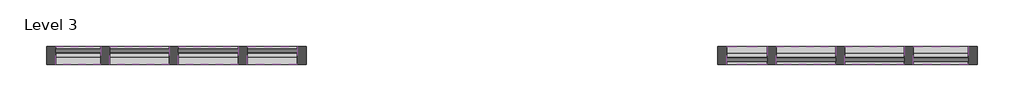
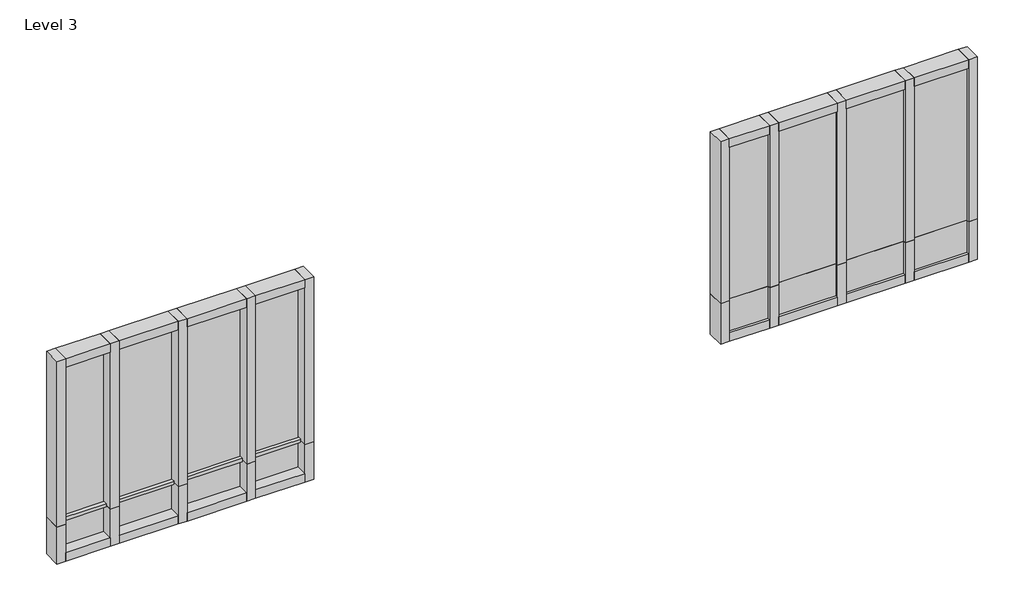
# One storey, incomplete: 44 members, 16 plates.
"""IFC4 building model written with IfcOpenShell, lengths in millimetres."""

from ifc_helpers import new_model, si_unit, origin, place, context, project, spatial, transform, mapped, element, save
from components import member_2ec808cb, member_7ddf0b01, member_ff98d70f, member_bdd069ac, member_fa046a42, member_66d82eec, member_4918008d, member_3060f3e2, member_6be37683, member_ccaabd6e, member_6ea553f1, member_a1da5be3, member_71eb4692, member_d3323a85, member_6c34f49c, member_dffdf235, member_75d1e245, member_2b49869a, member_75074519, member_3c3dc66a, system_panel_glazed_5633d65b, system_panel_glazed_b006000b, system_panel_glazed_54f7da7e, system_panel_glazed_325805c1, system_panel_glazed_de0a1ab2, system_panel_glazed_75a4b6fa, system_panel_glazed_925bd09e, system_panel_glazed_45aa6f3c, system_panel_glazed_e947191b, system_panel_glazed_5768b914, system_panel_glazed_0f3faf12, system_panel_glazed_eddfd4ea, system_panel_glazed_fe17e9eb, system_panel_glazed_f0550140

model = new_model("IFC4")

# Units and contexts
model_context = context("Model", 3, world=origin())
ifc_project = project(units=[si_unit("LENGTHUNIT", "METRE", prefix="MILLI")], contexts=[model_context])

# Site, building, storey
site = spatial("IfcSite", under=ifc_project)
building = spatial("IfcBuilding", under=site)
storey = spatial("IfcBuildingStorey", under=building, Name="Level 3", Elevation=3200.4)

# Members
placement = place(None, origin())
member_shape = member_2ec808cb(model_context)
element("IfcMember", 1, ObjectType="Rectangular Mullion : 1\" Square", at=placement, inside=storey, context=model_context, shape_type="MappedRepresentation", body=[
    mapped(member_shape, transform((-4793.1680265, 1641.9286055, 4089.4), x_axis=(0.0, 0.0, 1.0), y_axis=(0.0, -1.0, 0.0), z_axis=(1.0, 0.0, 0.0))),
])
member_2_shape = member_7ddf0b01(model_context)
element("IfcMember", 2, ObjectType="Rectangular Mullion : 1\" Square", at=placement, inside=storey, context=model_context, shape_type="MappedRepresentation", body=[
    mapped(member_2_shape, transform((-5208.0346932, 1641.9286055, 4089.4), x_axis=(0.0, 0.0, 1.0), y_axis=(0.0, -1.0, 0.0), z_axis=(1.0, 0.0, 0.0))),
])
member_3_shape = member_ff98d70f(model_context)
element("IfcMember", 3, ObjectType="Rectangular Mullion : 1\" Square", at=placement, inside=storey, context=model_context, shape_type="MappedRepresentation", body=[
    mapped(member_3_shape, transform((-5694.8680265, 1641.9286055, 4089.4), x_axis=(0.0, 0.0, 1.0), y_axis=(0.0, -1.0, 0.0), z_axis=(1.0, 0.0, 0.0))),
])
element("IfcMember", 4, ObjectType="Rectangular Mullion : 1\" Square", at=placement, inside=storey, context=model_context, shape_type="MappedRepresentation", body=[
    mapped(member_3_shape, transform((-938.7180265, 1641.9286055, 4114.8), x_axis=(0.0, 0.0, 1.0), y_axis=(0.0, 1.0, 0.0), z_axis=(-1.0, 0.0, 0.0))),
])
element("IfcMember", 5, ObjectType="Rectangular Mullion : 1\" Square", at=placement, inside=storey, context=model_context, shape_type="MappedRepresentation", body=[
    mapped(member_3_shape, transform((-1421.3180265, 1641.9286055, 4114.8), x_axis=(0.0, 0.0, 1.0), y_axis=(0.0, 1.0, 0.0), z_axis=(-1.0, 0.0, 0.0))),
])
member_4_shape = member_bdd069ac(model_context)
element("IfcMember", 6, ObjectType="Rectangular Mullion : 1\" Square", at=placement, inside=storey, context=model_context, shape_type="MappedRepresentation", body=[
    mapped(member_4_shape, transform((-6177.4680265, 1641.9286055, 4089.4), x_axis=(0.0, 0.0, 1.0), y_axis=(0.0, -1.0, 0.0), z_axis=(1.0, 0.0, 0.0))),
])
member_5_shape = member_fa046a42(model_context)
element("IfcMember", 7, ObjectType="Rectangular Mullion : 1\" Square", at=placement, inside=storey, context=model_context, shape_type="MappedRepresentation", body=[
    mapped(member_5_shape, transform((-1770.5680265, 1641.9286055, 4114.8), x_axis=(0.0, 0.0, 1.0), y_axis=(0.0, 1.0, 0.0), z_axis=(-1.0, 0.0, 0.0))),
])
member_6_shape = member_66d82eec(model_context)
element("IfcMember", 8, ObjectType="Rectangular Mullion : 1\" Square", at=placement, inside=storey, context=model_context, shape_type="MappedRepresentation", body=[
    mapped(member_6_shape, transform((-456.1180265, 1641.9286055, 4114.8), x_axis=(0.0, 0.0, 1.0), y_axis=(0.0, 1.0, 0.0), z_axis=(-1.0, 0.0, 0.0))),
])
member_7_shape = member_4918008d(model_context)
element("IfcMember", 9, ObjectType="Rectangular Mullion : 2.5\" x 5\" rectangular", at=placement, inside=storey, context=model_context, shape_type="MappedRepresentation", body=[
    mapped(member_7_shape, transform((-4793.1680265, 1641.9286055, 5334.0), x_axis=(0.0, 0.0, 1.0), y_axis=(0.0, -1.0, 0.0), z_axis=(1.0, 0.0, 0.0))),
])
member_8_shape = member_3060f3e2(model_context)
element("IfcMember", 10, ObjectType="Rectangular Mullion : 2.5\" x 5\" rectangular", at=placement, inside=storey, context=model_context, shape_type="MappedRepresentation", body=[
    mapped(member_8_shape, transform((-6494.9680265, 1641.9286055, 3810.0), x_axis=(0.0, 0.0, -1.0), y_axis=(0.0, -1.0, 0.0), z_axis=(-1.0, 0.0, 0.0))),
])
member_9_shape = member_6be37683(model_context)
element("IfcMember", 11, ObjectType="Rectangular Mullion : 2.5\" x 5\" rectangular", at=placement, inside=storey, context=model_context, shape_type="MappedRepresentation", body=[
    mapped(member_9_shape, transform((-6145.7180265, 1641.9286055, 3810.0), x_axis=(1.0, 0.0, 0.0), y_axis=(0.0, -1.0, 0.0), z_axis=(0.0, 0.0, -1.0))),
])
element("IfcMember", 12, ObjectType="Rectangular Mullion : 2.5\" x 5\" rectangular", at=placement, inside=storey, context=model_context, shape_type="MappedRepresentation", body=[
    mapped(member_9_shape, transform((-5663.1180265, 1641.9286055, 3810.0), x_axis=(1.0, 0.0, 0.0), y_axis=(0.0, -1.0, 0.0), z_axis=(0.0, 0.0, -1.0))),
])
element("IfcMember", 13, ObjectType="Rectangular Mullion : 2.5\" x 5\" rectangular", at=placement, inside=storey, context=model_context, shape_type="MappedRepresentation", body=[
    mapped(member_9_shape, transform((-5176.2846932, 1641.9286055, 3810.0), x_axis=(1.0, 0.0, 0.0), y_axis=(0.0, -1.0, 0.0), z_axis=(0.0, 0.0, -1.0))),
])
member_10_shape = member_ccaabd6e(model_context)
element("IfcMember", 14, ObjectType="Rectangular Mullion : 2.5\" x 5\" rectangular", at=placement, inside=storey, context=model_context, shape_type="MappedRepresentation", body=[
    mapped(member_10_shape, transform((-6113.9680265, 1641.9286055, 3810.0), x_axis=(0.0, 0.0, -1.0), y_axis=(0.0, -1.0, 0.0), z_axis=(-1.0, 0.0, 0.0))),
])
element("IfcMember", 15, ObjectType="Rectangular Mullion : 2.5\" x 5\" rectangular", at=placement, inside=storey, context=model_context, shape_type="MappedRepresentation", body=[
    mapped(member_10_shape, transform((-1002.2180265, 1641.9286055, 3810.0), x_axis=(0.0, 0.0, -1.0), y_axis=(0.0, 1.0, 0.0), z_axis=(1.0, 0.0, 0.0))),
])
element("IfcMember", 16, ObjectType="Rectangular Mullion : 2.5\" x 5\" rectangular", at=placement, inside=storey, context=model_context, shape_type="MappedRepresentation", body=[
    mapped(member_10_shape, transform((-519.6180265, 1641.9286055, 3810.0), x_axis=(0.0, 0.0, -1.0), y_axis=(0.0, 1.0, 0.0), z_axis=(1.0, 0.0, 0.0))),
])
member_11_shape = member_6ea553f1(model_context)
element("IfcMember", 17, ObjectType="Rectangular Mullion : 2.5\" x 5\" rectangular", at=placement, inside=storey, context=model_context, shape_type="MappedRepresentation", body=[
    mapped(member_11_shape, transform((-5631.3680265, 1641.9286055, 3810.0), x_axis=(0.0, 0.0, -1.0), y_axis=(0.0, -1.0, 0.0), z_axis=(-1.0, 0.0, 0.0))),
])
element("IfcMember", 18, ObjectType="Rectangular Mullion : 2.5\" x 5\" rectangular", at=placement, inside=storey, context=model_context, shape_type="MappedRepresentation", body=[
    mapped(member_7_shape, transform((-5144.5346932, 1641.9286055, 3810.0), x_axis=(0.0, 0.0, -1.0), y_axis=(0.0, -1.0, 0.0), z_axis=(-1.0, 0.0, 0.0))),
])
element("IfcMember", 19, ObjectType="Rectangular Mullion : 2.5\" x 5\" rectangular", at=placement, inside=storey, context=model_context, shape_type="MappedRepresentation", body=[
    mapped(member_8_shape, transform((-6177.4680265, 1641.9286055, 5334.0), x_axis=(0.0, 0.0, 1.0), y_axis=(0.0, -1.0, 0.0), z_axis=(1.0, 0.0, 0.0))),
])
element("IfcMember", 20, ObjectType="Rectangular Mullion : 2.5\" x 5\" rectangular", at=placement, inside=storey, context=model_context, shape_type="MappedRepresentation", body=[
    mapped(member_10_shape, transform((-5694.8680265, 1641.9286055, 5334.0), x_axis=(0.0, 0.0, 1.0), y_axis=(0.0, -1.0, 0.0), z_axis=(1.0, 0.0, 0.0))),
])
element("IfcMember", 21, ObjectType="Rectangular Mullion : 2.5\" x 5\" rectangular", at=placement, inside=storey, context=model_context, shape_type="MappedRepresentation", body=[
    mapped(member_10_shape, transform((-1421.3180265, 1641.9286055, 5334.0), x_axis=(0.0, 0.0, 1.0), y_axis=(0.0, 1.0, 0.0), z_axis=(-1.0, 0.0, 0.0))),
])
element("IfcMember", 22, ObjectType="Rectangular Mullion : 2.5\" x 5\" rectangular", at=placement, inside=storey, context=model_context, shape_type="MappedRepresentation", body=[
    mapped(member_10_shape, transform((-938.7180265, 1641.9286055, 5334.0), x_axis=(0.0, 0.0, 1.0), y_axis=(0.0, 1.0, 0.0), z_axis=(-1.0, 0.0, 0.0))),
])
element("IfcMember", 23, ObjectType="Rectangular Mullion : 2.5\" x 5\" rectangular", at=placement, inside=storey, context=model_context, shape_type="MappedRepresentation", body=[
    mapped(member_11_shape, transform((-5208.0346932, 1641.9286055, 5334.0), x_axis=(0.0, 0.0, 1.0), y_axis=(0.0, -1.0, 0.0), z_axis=(1.0, 0.0, 0.0))),
])
member_12_shape = member_a1da5be3(model_context)
element("IfcMember", 24, ObjectType="Rectangular Mullion : 2.5\" x 5\" rectangular", at=placement, inside=storey, context=model_context, shape_type="MappedRepresentation", body=[
    mapped(member_12_shape, transform((-6145.7180265, 1641.9286055, 4089.4), x_axis=(1.0, 0.0, 0.0), y_axis=(0.0, -1.0, 0.0), z_axis=(0.0, 0.0, -1.0))),
])
element("IfcMember", 25, ObjectType="Rectangular Mullion : 2.5\" x 5\" rectangular", at=placement, inside=storey, context=model_context, shape_type="MappedRepresentation", body=[
    mapped(member_12_shape, transform((-5663.1180265, 1641.9286055, 4089.4), x_axis=(1.0, 0.0, 0.0), y_axis=(0.0, -1.0, 0.0), z_axis=(0.0, 0.0, -1.0))),
])
element("IfcMember", 26, ObjectType="Rectangular Mullion : 2.5\" x 5\" rectangular", at=placement, inside=storey, context=model_context, shape_type="MappedRepresentation", body=[
    mapped(member_12_shape, transform((-5176.2846932, 1641.9286055, 4089.4), x_axis=(1.0, 0.0, 0.0), y_axis=(0.0, -1.0, 0.0), z_axis=(0.0, 0.0, -1.0))),
])
member_13_shape = member_71eb4692(model_context)
element("IfcMember", 27, ObjectType="Rectangular Mullion : 2.5\" x 5\" rectangular", at=placement, inside=storey, context=model_context, shape_type="MappedRepresentation", body=[
    mapped(member_13_shape, transform((-6558.4680265, 1641.9286055, 5334.0), x_axis=(-1.0, 0.0, 0.0), y_axis=(0.0, -1.0, 0.0), z_axis=(0.0, 0.0, 1.0))),
])
member_14_shape = member_d3323a85(model_context)
element("IfcMember", 28, ObjectType="Rectangular Mullion : 2.5\" x 5\" rectangular", at=placement, inside=storey, context=model_context, shape_type="MappedRepresentation", body=[
    mapped(member_14_shape, transform((-4729.6680265, 1641.9286055, 3810.0), x_axis=(1.0, 0.0, 0.0), y_axis=(0.0, -1.0, 0.0), z_axis=(0.0, 0.0, -1.0))),
])
element("IfcMember", 29, ObjectType="Rectangular Mullion : 2.5\" x 5\" rectangular", at=placement, inside=storey, context=model_context, shape_type="MappedRepresentation", body=[
    mapped(member_13_shape, transform((-4729.6680265, 1641.9286055, 4089.4), x_axis=(1.0, 0.0, 0.0), y_axis=(0.0, -1.0, 0.0), z_axis=(0.0, 0.0, -1.0))),
])
element("IfcMember", 30, ObjectType="Rectangular Mullion : 2.5\" x 5\" rectangular", at=placement, inside=storey, context=model_context, shape_type="MappedRepresentation", body=[
    mapped(member_14_shape, transform((-6558.4680265, 1641.9286055, 4089.4), x_axis=(-1.0, 0.0, 0.0), y_axis=(0.0, -1.0, 0.0), z_axis=(0.0, 0.0, 1.0))),
])
member_15_shape = member_6c34f49c(model_context)
element("IfcMember", 31, ObjectType="Rectangular Mullion : 2.5\" x 5\" rectangular", at=placement, inside=storey, context=model_context, shape_type="MappedRepresentation", body=[
    mapped(member_15_shape, transform((-1770.5680265, 1641.9286055, 5334.0), x_axis=(0.0, 0.0, 1.0), y_axis=(0.0, 1.0, 0.0), z_axis=(-1.0, 0.0, 0.0))),
])
member_16_shape = member_dffdf235(model_context)
element("IfcMember", 32, ObjectType="Rectangular Mullion : 2.5\" x 5\" rectangular", at=placement, inside=storey, context=model_context, shape_type="MappedRepresentation", body=[
    mapped(member_16_shape, transform((-68.7680265, 1641.9286055, 3810.0), x_axis=(0.0, 0.0, -1.0), y_axis=(0.0, 1.0, 0.0), z_axis=(1.0, 0.0, 0.0))),
])
member_17_shape = member_75d1e245(model_context)
element("IfcMember", 33, ObjectType="Rectangular Mullion : 2.5\" x 5\" rectangular", at=placement, inside=storey, context=model_context, shape_type="MappedRepresentation", body=[
    mapped(member_17_shape, transform((-1453.0680265, 1641.9286055, 3810.0), x_axis=(-1.0, 0.0, 0.0), y_axis=(0.0, 1.0, 0.0), z_axis=(0.0, 0.0, -1.0))),
])
element("IfcMember", 34, ObjectType="Rectangular Mullion : 2.5\" x 5\" rectangular", at=placement, inside=storey, context=model_context, shape_type="MappedRepresentation", body=[
    mapped(member_17_shape, transform((-970.4680265, 1641.9286055, 3810.0), x_axis=(-1.0, 0.0, 0.0), y_axis=(0.0, 1.0, 0.0), z_axis=(0.0, 0.0, -1.0))),
])
element("IfcMember", 35, ObjectType="Rectangular Mullion : 2.5\" x 5\" rectangular", at=placement, inside=storey, context=model_context, shape_type="MappedRepresentation", body=[
    mapped(member_17_shape, transform((-487.8680265, 1641.9286055, 3810.0), x_axis=(-1.0, 0.0, 0.0), y_axis=(0.0, 1.0, 0.0), z_axis=(0.0, 0.0, -1.0))),
])
element("IfcMember", 36, ObjectType="Rectangular Mullion : 2.5\" x 5\" rectangular", at=placement, inside=storey, context=model_context, shape_type="MappedRepresentation", body=[
    mapped(member_15_shape, transform((-1484.8180265, 1641.9286055, 3810.0), x_axis=(0.0, 0.0, -1.0), y_axis=(0.0, 1.0, 0.0), z_axis=(1.0, 0.0, 0.0))),
])
element("IfcMember", 37, ObjectType="Rectangular Mullion : 2.5\" x 5\" rectangular", at=placement, inside=storey, context=model_context, shape_type="MappedRepresentation", body=[
    mapped(member_16_shape, transform((-456.1180265, 1641.9286055, 5334.0), x_axis=(0.0, 0.0, 1.0), y_axis=(0.0, 1.0, 0.0), z_axis=(-1.0, 0.0, 0.0))),
])
member_18_shape = member_2b49869a(model_context)
element("IfcMember", 38, ObjectType="Rectangular Mullion : 2.5\" x 5\" rectangular", at=placement, inside=storey, context=model_context, shape_type="MappedRepresentation", body=[
    mapped(member_18_shape, transform((-1453.0680265, 1641.9286055, 4114.8), x_axis=(-1.0, 0.0, 0.0), y_axis=(0.0, 1.0, 0.0), z_axis=(0.0, 0.0, -1.0))),
])
element("IfcMember", 39, ObjectType="Rectangular Mullion : 2.5\" x 5\" rectangular", at=placement, inside=storey, context=model_context, shape_type="MappedRepresentation", body=[
    mapped(member_18_shape, transform((-970.4680265, 1641.9286055, 4114.8), x_axis=(-1.0, 0.0, 0.0), y_axis=(0.0, 1.0, 0.0), z_axis=(0.0, 0.0, -1.0))),
])
element("IfcMember", 40, ObjectType="Rectangular Mullion : 2.5\" x 5\" rectangular", at=placement, inside=storey, context=model_context, shape_type="MappedRepresentation", body=[
    mapped(member_18_shape, transform((-487.8680265, 1641.9286055, 4114.8), x_axis=(-1.0, 0.0, 0.0), y_axis=(0.0, 1.0, 0.0), z_axis=(0.0, 0.0, -1.0))),
])
member_19_shape = member_75074519(model_context)
element("IfcMember", 41, ObjectType="Rectangular Mullion : 2.5\" x 5\" rectangular", at=placement, inside=storey, context=model_context, shape_type="MappedRepresentation", body=[
    mapped(member_19_shape, transform((-5.2680265, 1641.9286055, 5334.0), x_axis=(1.0, 0.0, 0.0), y_axis=(0.0, 1.0, 0.0), z_axis=(0.0, 0.0, 1.0))),
])
member_20_shape = member_3c3dc66a(model_context)
element("IfcMember", 42, ObjectType="Rectangular Mullion : 2.5\" x 5\" rectangular", at=placement, inside=storey, context=model_context, shape_type="MappedRepresentation", body=[
    mapped(member_20_shape, transform((-1834.0680265, 1641.9286055, 3810.0), x_axis=(-1.0, 0.0, 0.0), y_axis=(0.0, 1.0, 0.0), z_axis=(0.0, 0.0, -1.0))),
])
element("IfcMember", 43, ObjectType="Rectangular Mullion : 2.5\" x 5\" rectangular", at=placement, inside=storey, context=model_context, shape_type="MappedRepresentation", body=[
    mapped(member_19_shape, transform((-1834.0680265, 1641.9286055, 4114.8), x_axis=(-1.0, 0.0, 0.0), y_axis=(0.0, 1.0, 0.0), z_axis=(0.0, 0.0, -1.0))),
])
element("IfcMember", 44, ObjectType="Rectangular Mullion : 2.5\" x 5\" rectangular", at=placement, inside=storey, context=model_context, shape_type="MappedRepresentation", body=[
    mapped(member_20_shape, transform((-5.2680265, 1641.9286055, 4114.8), x_axis=(1.0, 0.0, 0.0), y_axis=(0.0, 1.0, 0.0), z_axis=(0.0, 0.0, 1.0))),
])

# Plates
system_panel_glazed_shape = system_panel_glazed_5633d65b(model_context)
element("IfcPlate", 45, ObjectType="System Panel : Glazed", at=placement, inside=storey, context=model_context, shape_type="MappedRepresentation", body=[
    mapped(system_panel_glazed_shape, transform((-6336.2180265, 1641.9286055, 3873.5), x_axis=(1.0, 0.0, 0.0), y_axis=(0.0, 1.0, 0.0), z_axis=(0.0, 0.0, 1.0))),
])
system_panel_glazed_2_shape = system_panel_glazed_b006000b(model_context)
element("IfcPlate", 46, ObjectType="System Panel : Glazed", at=placement, inside=storey, context=model_context, shape_type="MappedRepresentation", body=[
    mapped(system_panel_glazed_2_shape, transform((-5904.4180265, 1641.9286055, 3873.5), x_axis=(1.0, 0.0, 0.0), y_axis=(0.0, 1.0, 0.0), z_axis=(0.0, 0.0, 1.0))),
])
system_panel_glazed_3_shape = system_panel_glazed_54f7da7e(model_context)
element("IfcPlate", 47, ObjectType="System Panel : Glazed", at=placement, inside=storey, context=model_context, shape_type="MappedRepresentation", body=[
    mapped(system_panel_glazed_3_shape, transform((-5419.7013599, 1641.9286055, 3873.5), x_axis=(1.0, 0.0, 0.0), y_axis=(0.0, 1.0, 0.0), z_axis=(0.0, 0.0, 1.0))),
])
system_panel_glazed_4_shape = system_panel_glazed_325805c1(model_context)
element("IfcPlate", 48, ObjectType="System Panel : Glazed", at=placement, inside=storey, context=model_context, shape_type="MappedRepresentation", body=[
    mapped(system_panel_glazed_4_shape, transform((-4968.8513599, 1641.9286055, 3873.5), x_axis=(1.0, 0.0, 0.0), y_axis=(0.0, 1.0, 0.0), z_axis=(0.0, 0.0, 1.0))),
])
system_panel_glazed_5_shape = system_panel_glazed_de0a1ab2(model_context)
element("IfcPlate", 49, ObjectType="System Panel : Glazed", at=placement, inside=storey, context=model_context, shape_type="MappedRepresentation", body=[
    mapped(system_panel_glazed_5_shape, transform((-6336.2180265, 1641.9286055, 4089.4), x_axis=(1.0, 0.0, 0.0), y_axis=(0.0, 1.0, 0.0), z_axis=(0.0, 0.0, 1.0))),
])
system_panel_glazed_6_shape = system_panel_glazed_75a4b6fa(model_context)
element("IfcPlate", 50, ObjectType="System Panel : Glazed", at=placement, inside=storey, context=model_context, shape_type="MappedRepresentation", body=[
    mapped(system_panel_glazed_6_shape, transform((-5904.4180265, 1641.9286055, 4089.4), x_axis=(1.0, 0.0, 0.0), y_axis=(0.0, 1.0, 0.0), z_axis=(0.0, 0.0, 1.0))),
])
system_panel_glazed_7_shape = system_panel_glazed_925bd09e(model_context)
element("IfcPlate", 51, ObjectType="System Panel : Glazed", at=placement, inside=storey, context=model_context, shape_type="MappedRepresentation", body=[
    mapped(system_panel_glazed_7_shape, transform((-5419.7013599, 1641.9286055, 4089.4), x_axis=(1.0, 0.0, 0.0), y_axis=(0.0, 1.0, 0.0), z_axis=(0.0, 0.0, 1.0))),
])
system_panel_glazed_8_shape = system_panel_glazed_45aa6f3c(model_context)
element("IfcPlate", 52, ObjectType="System Panel : Glazed", at=placement, inside=storey, context=model_context, shape_type="MappedRepresentation", body=[
    mapped(system_panel_glazed_8_shape, transform((-4968.8513599, 1641.9286055, 4089.4), x_axis=(1.0, 0.0, 0.0), y_axis=(0.0, 1.0, 0.0), z_axis=(0.0, 0.0, 1.0))),
])
system_panel_glazed_9_shape = system_panel_glazed_e947191b(model_context)
element("IfcPlate", 53, ObjectType="System Panel : Glazed", at=placement, inside=storey, context=model_context, shape_type="MappedRepresentation", body=[
    mapped(system_panel_glazed_9_shape, transform((-262.4430265, 1641.9286055, 3873.5), x_axis=(-1.0, 0.0, 0.0), y_axis=(0.0, -1.0, 0.0), z_axis=(0.0, 0.0, 1.0))),
])
system_panel_glazed_10_shape = system_panel_glazed_5768b914(model_context)
element("IfcPlate", 54, ObjectType="System Panel : Glazed", at=placement, inside=storey, context=model_context, shape_type="MappedRepresentation", body=[
    mapped(system_panel_glazed_10_shape, transform((-1627.6930265, 1641.9286055, 3873.5), x_axis=(-1.0, 0.0, 0.0), y_axis=(0.0, -1.0, 0.0), z_axis=(0.0, 0.0, 1.0))),
])
system_panel_glazed_11_shape = system_panel_glazed_0f3faf12(model_context)
element("IfcPlate", 55, ObjectType="System Panel : Glazed", at=placement, inside=storey, context=model_context, shape_type="MappedRepresentation", body=[
    mapped(system_panel_glazed_11_shape, transform((-1211.7680265, 1641.9286055, 3873.5), x_axis=(-1.0, 0.0, 0.0), y_axis=(0.0, -1.0, 0.0), z_axis=(0.0, 0.0, 1.0))),
])
element("IfcPlate", 56, ObjectType="System Panel : Glazed", at=placement, inside=storey, context=model_context, shape_type="MappedRepresentation", body=[
    mapped(system_panel_glazed_11_shape, transform((-729.1680265, 1641.9286055, 3873.5), x_axis=(-1.0, 0.0, 0.0), y_axis=(0.0, -1.0, 0.0), z_axis=(0.0, 0.0, 1.0))),
])
system_panel_glazed_12_shape = system_panel_glazed_eddfd4ea(model_context)
element("IfcPlate", 57, ObjectType="System Panel : Glazed", at=placement, inside=storey, context=model_context, shape_type="MappedRepresentation", body=[
    mapped(system_panel_glazed_12_shape, transform((-262.4430265, 1641.9286055, 4114.8), x_axis=(-1.0, 0.0, 0.0), y_axis=(0.0, -1.0, 0.0), z_axis=(0.0, 0.0, 1.0))),
])
system_panel_glazed_13_shape = system_panel_glazed_fe17e9eb(model_context)
element("IfcPlate", 58, ObjectType="System Panel : Glazed", at=placement, inside=storey, context=model_context, shape_type="MappedRepresentation", body=[
    mapped(system_panel_glazed_13_shape, transform((-729.1680265, 1641.9286055, 4114.8), x_axis=(-1.0, 0.0, 0.0), y_axis=(0.0, -1.0, 0.0), z_axis=(0.0, 0.0, 1.0))),
])
element("IfcPlate", 59, ObjectType="System Panel : Glazed", at=placement, inside=storey, context=model_context, shape_type="MappedRepresentation", body=[
    mapped(system_panel_glazed_13_shape, transform((-1211.7680265, 1641.9286055, 4114.8), x_axis=(-1.0, 0.0, 0.0), y_axis=(0.0, -1.0, 0.0), z_axis=(0.0, 0.0, 1.0))),
])
system_panel_glazed_14_shape = system_panel_glazed_f0550140(model_context)
element("IfcPlate", 60, ObjectType="System Panel : Glazed", at=placement, inside=storey, context=model_context, shape_type="MappedRepresentation", body=[
    mapped(system_panel_glazed_14_shape, transform((-1627.6930265, 1641.9286055, 4114.8), x_axis=(-1.0, 0.0, 0.0), y_axis=(0.0, -1.0, 0.0), z_axis=(0.0, 0.0, 1.0))),
])

save(model, "model.ifc")

# Revit data of these elements
# Type "Rectangular Mullion : 1\" Square"
#   built-in parameter 1007304 = 0.0833333 (stored number, unit not read)
#   built-in parameter 1007301 = 0.0416667 (stored number, unit not read)
#   built-in parameter 1007300 = 0.0416667 (stored number, unit not read)
# Type "Rectangular Mullion : 2.5\" x 5\" rectangular"
#   built-in parameter 1007304 = 0.416667 (stored number, unit not read)
#   built-in parameter 1007301 = 0.104167 (stored number, unit not read)
#   built-in parameter 1007300 = 0.104167 (stored number, unit not read)
# Type "System Panel : Glazed"
#   Construction Type Id = "GSP4R"
#   Analytic Construction = "1/8 in Pilkington single glazing"
#   Visual Light Transmittance = 0.9
#   Solar Heat Gain Coefficient = 0.86
#   Heat Transfer Coefficient (U) = 1.18115 BTU/(h·ft²·°F)
#   Define Thermal Properties by = 1
# Elements 1, 2, 3, 4, 5, 6, 7, 8 (IfcMember, "Rectangular Mullion : 1\" Square")
#   Phase Created = New Construction
#   Materials on its faces: "Aluminum"
# Elements 9, 10, 11, 12, 13, 14, 15, 16, 17, 18, 19, 20, 21, 22, 23, 24, 25, 26, 27, 28, 29, 30, 31, 32, 33, 34, 35, 36, 37, 38, 39, 40, 41, 42, 43, 44 (IfcMember, "Rectangular Mullion : 2.5\" x 5\" rectangular")
#   Phase Created = New Construction
# Elements 45, 46, 47, 48, 49, 50, 51, 52, 53, 54, 55, 56, 57, 58, 59, 60 (IfcPlate, "System Panel : Glazed")
#   Phase Created = New Construction
#   Materials on its faces: "Glass"
# Materials
#   "Aluminum": class "Metal", colour RGB 247 247 247, transparency 0, Description = "Aluminum 6061", Cost = 0
#   "Glass": class "Glass", colour RGB 0 128 192, transparency 0.75, Description = "Soda Lime Glass", Cost = 0
